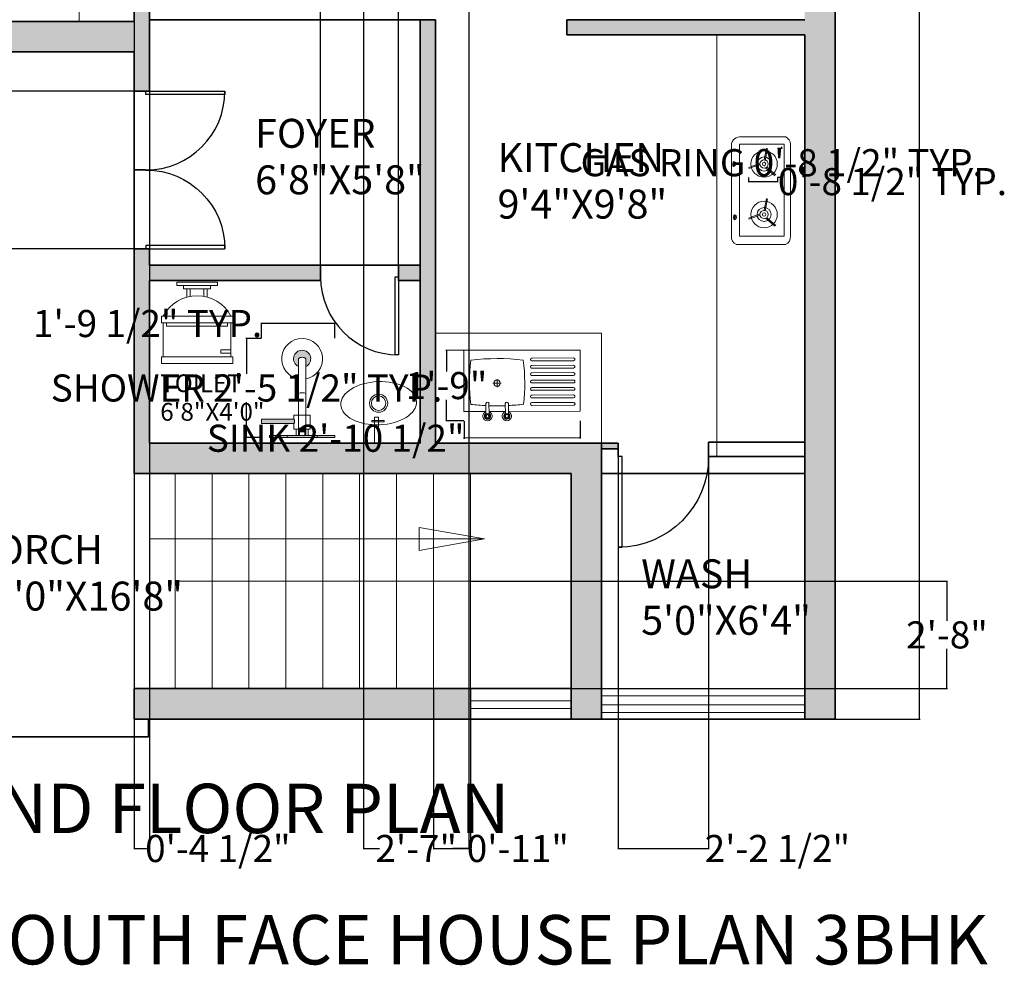
# Model space of a CAD drawing. Units: inches. Extents: x -4737294 to -4736756, y 1716389 to 1717040.
# Tile 16 of 25: x -4737096 to -4736805, y 1716389 to 1716669. Entities that reach past the tile are written whole.
import ezdxf

# ---------------------------------------------------------------- set-up
doc = ezdxf.new("R2010")
doc.units = ezdxf.units.IN
doc.header["$MEASUREMENT"] = 0
for name, color, linetype, lineweight in [('A-ANNO-DIMS', 2, 'Continuous', 18), ('A-ANNO-TEXT', 250, 'Continuous', 30), ('A-AREA-IDEN', 250, 'Continuous', 18), ('A-EQPM', 250, 'Continuous', 18), ('A-FLOR-CASE', 250, 'Continuous', 18), ('A-FLOR-STRS', 252, 'Continuous', 18), ('A-GLAZ', 4, 'Continuous', 18), ('A-WALL-PATT', 244, 'Continuous', 13), ('doors', 252, 'Continuous', 25), ('furniture', 250, 'Continuous', 18), ('PLUMBING FIXTURES', 252, 'Continuous', 18), ('walls', 252, 'Continuous', 35)]:
    doc.layers.add(name, color=color, linetype=linetype, lineweight=lineweight)
doc.styles.get("Standard").update_dxf_attribs({"font": 'arial.ttf'})
doc.dimstyles.get("Standard").update_dxf_attribs({"dimtxt": 8, "dimasz": 0.18, "dimexe": 0.18, "dimexo": 0.0625, "dimgap": 0.09, "dimtad": 0, "dimtih": 1, "dimtoh": 1, "dimzin": 0, "dimdsep": 46, "dimlunit": 3, "dimtxsty": 'Standard', "dimcen": 0.09, "dimadec": 0, "dimazin": 0, "dimtfac": 1, "dimtofl": 0, "dimtmove": 0, "dimatfit": 3, "dimfxl": 1, "dimtolj": 1, "dimtzin": 0, "dimarcsym": 0})

# ---------------------------------------------------------------- blocks, each defined once
blk = doc.blocks.new('*D22')
at = {"layer": 'A-ANNO-DIMS', "color": 0, "lineweight": -2, "transparency": 16777216}
for p, q in [((-4736855.08, 1717002.06), (-4736830.06, 1717002.06)), ((-4736830.24, 1717001.88), (-4736830.24, 1716736.22)), ((-4736830.24, 1716462.24), (-4736830.24, 1716727.91)), ((-4736855.08, 1716462.06), (-4736830.06, 1716462.06))]:
    blk.add_line(p, q, dxfattribs=at)
at = {"layer": 'A-ANNO-DIMS', "color": 0, "transparency": 16777216}
for points in [[(-4736830.27, 1717001.88), (-4736830.21, 1717001.88), (-4736830.24, 1717002.06)], [(-4736830.27, 1716462.24), (-4736830.21, 1716462.24), (-4736830.24, 1716462.06)]]:
    blk.add_solid(points, dxfattribs=at)
at = {"layer": 'Defpoints', "color": 0, "transparency": 16777216}
for p in [(-4736855.14, 1717002.06), (-4736830.24, 1717002.06), (-4736855.14, 1716462.06)]:
    blk.add_point(p, dxfattribs=at)
at = {"layer": 'A-ANNO-DIMS', "color": 0, "transparency": 16777216, "insert": (-4736830.24, 1716732.06), "char_height": 8, "attachment_point": 5}
blk.add_mtext("\\A1;45'", dxfattribs=at)
blk = doc.blocks.new('A$C799204C7')
for p, q in [((0, 34.2), (17.99, 34.2)), ((0, 0), (0, 34.2)), ((2.32, 20.01), (2.32, 32.27)), ((3.13, 20.01), (3.13, 32.27)), ((4.48, 20.01), (4.48, 32.27)), ((5.29, 20.01), (5.29, 32.27)), ((6.64, 20.01), (6.64, 32.27)), ((7.45, 20.01), (7.45, 32.27)), ((8.85, 20.01), (8.85, 32.27)), ((9.66, 20.01), (9.66, 32.27)), ((11.01, 20.01), (11.01, 32.27)), ((11.82, 20.01), (11.82, 32.27)), ((13.22, 20.01), (13.22, 32.27)), ((14.03, 20.01), (14.03, 32.27)), ((15.42, 20.01), (15.42, 32.27)), ((16.24, 20.01), (16.24, 32.27)), ((17.99, 13.08), (17.99, 34.2)), ((18.59, 13.08), (15.71, 13.08)), ((15.71, 12.17), (18.59, 12.17)), ((17.99, 7.36), (17.99, 12.17)), ((8.52, 9.77), (10.9, 9.77)), ((9.73, 11), (9.73, 8.54)), ((18.59, 7.36), (15.71, 7.36)), ((15.71, 6.45), (18.59, 6.45)), ((17.99, 0), (17.99, 6.45)), ((0, 0), (17.99, 0))]:
    blk.add_line(p, q)
for centre, radius in [((19.38, 12.62), 0.684), ((19.38, 12.62), 0.456), ((9.7, 9.77), 0.916), ((19.38, 6.91), 0.684), ((19.38, 6.91), 0.456)]:
    blk.add_circle(centre, radius)
for centre, radius, start, end in [((2.72, 32.27), 0.407, 0, 180), ((4.88, 32.27), 0.407, 0, 180), ((7.05, 32.27), 0.407, 0, 180), ((9.25, 32.27), 0.407, 0, 180), ((11.42, 32.27), 0.407, 0, 180), ((13.62, 32.27), 0.407, 0, 180), ((15.83, 32.27), 0.407, 0, 180), ((2.72, 20.01), 0.407, 180, 0), ((67.33, 9.77), 64.88, 173.1952, 186.8048), ((9.53, -30.19), 48.1, 82.3437, 97.8966), ((4.88, 20.01), 0.407, 180, 0), ((7.05, 20.01), 0.407, 180, 0), ((9.25, 20.01), 0.407, 180, 0), ((11.42, 20.01), 0.407, 180, 0), ((13.62, 20.01), 0.407, 180, 0), ((15.83, 20.01), 0.407, 180, 0), ((-48.51, 9.77), 64.88, 2.9208, 6.8048), ((15.71, 12.62), 0.456, 90, 270), ((-48.51, 9.77), 64.88, 357.8723, 2.115), ((19.38, 12.62), 1.37, 199.6514, 160.3603), ((19.38, 12.62), 0.911, 210.3431, 149.7554), ((15.71, 6.91), 0.456, 90, 270), ((-48.51, 9.77), 64.88, 353.1952, 357.0665), ((19.38, 6.91), 1.37, 199.6514, 160.3603), ((19.38, 6.91), 0.911, 210.3431, 149.7554), ((9.53, 49.73), 48.1, 262.1034, 277.6563)]:
    blk.add_arc(centre, radius, start, end)
blk = doc.blocks.new('sink')
at = {"layer": 'furniture'}
for p, q in [((8718164202.684322, -1433730581.131674), (8718164202.684322, -1433730583.598095)), ((8718164203.894819, -1433730582.369047), (8718164201.504578, -1433730582.369047)), ((8718164196.150837, -1433730592.638258), (8718164196.150837, -1433730604.938997)), ((8718164196.967728, -1433730592.638258), (8718164196.967728, -1433730604.938997)), ((8718164198.365185, -1433730592.638258), (8718164198.365185, -1433730604.938997)), ((8718164199.182076, -1433730592.638258), (8718164199.182076, -1433730604.938997)), ((8718164200.579533, -1433730592.638258), (8718164200.579533, -1433730604.938997)), ((8718164201.396423, -1433730592.638258), (8718164201.396423, -1433730604.938997)), ((8718164202.748692, -1433730592.638258), (8718164202.748692, -1433730604.938997)), ((8718164203.565582, -1433730592.638258), (8718164203.565582, -1433730604.938997)), ((8718164204.963041, -1433730592.638258), (8718164204.963041, -1433730604.938997)), ((8718164205.779934, -1433730592.638258), (8718164205.779934, -1433730604.938997)), ((8718164207.1322, -1433730592.638258), (8718164207.1322, -1433730604.938997)), ((8718164207.949093, -1433730592.638258), (8718164207.949093, -1433730604.938997)), ((8718164209.301359, -1433730592.638258), (8718164209.301359, -1433730604.938997)), ((8718164210.118252, -1433730592.638258), (8718164210.118252, -1433730604.938997))]:
    blk.add_line(p, q, dxfattribs=at)
for centre, radius in [((8718164192.998869, -1433730579.495552), 0.685789), ((8718164192.998869, -1433730579.495552), 0.457192), ((8718164202.715019, -1433730582.369047), 0.919003), ((8718164192.998869, -1433730585.228166), 0.68579), ((8718164192.998869, -1433730585.228166), 0.68579), ((8718164192.998869, -1433730585.228166), 0.457192)]:
    blk.add_circle(centre, radius, dxfattribs=at)
for centre, radius, start, end in [((8718164196.559284, -1433730592.638258), 0.41045, 354.3355999, 185.6644001), ((8718164198.77363, -1433730592.638258), 0.41045, 354.3355999, 185.6644001), ((8718164200.98798, -1433730592.638258), 0.41045, 354.3355999, 185.6644001), ((8718164203.157139, -1433730592.638258), 0.41045, 354.3355999, 185.6644001), ((8718164205.371487, -1433730592.638258), 0.41045, 354.3355999, 185.6644001), ((8718164207.540646, -1433730592.640262), 0.41045, 354.3355999, 185.6644001), ((8718164209.709805, -1433730592.640262), 0.41045, 354.3355999, 185.6644001), ((8718164196.559284, -1433730604.938997), 0.408445, 180, 0), ((8718164198.77363, -1433730604.938997), 0.408445, 180, 0), ((8718164200.98798, -1433730604.938997), 0.408445, 180, 0), ((8718164203.157139, -1433730604.938997), 0.408445, 180, 0), ((8718164205.371487, -1433730604.938997), 0.408445, 180, 0), ((8718164207.540646, -1433730604.938997), 0.408445, 180, 0), ((8718164209.709805, -1433730604.938997), 0.408445, 180, 0)]:
    blk.add_arc(centre, radius, start, end, dxfattribs=at)
at = {"layer": 'furniture', "xscale": 1.0032, "yscale": 1.0032, "zscale": 1.0032, "rotation": 180}
blk.add_blockref('A$C799204C7', (8718164212.441259, -1433730572.566334), dxfattribs=at)
blk = doc.blocks.new('washbasin')
at = {"layer": 'furniture'}
blk.add_blockref('sink', (-8718164214.119328, 1433730589.721069), dxfattribs=at)
blk = doc.blocks.new('O.H SHOWER-PL')
at = {"layer": 'PLUMBING FIXTURES'}
for points in [[(-1.84, 0), (-1.84, -0.25), (1.84, -0.25), (1.84, 0)], [(0.46, -8.72), (0.46, -9.67, -0.422337), (-0.46, -9.67), (-0.46, -8.72, 4.325472)]]:
    blk.add_hatch(color=256, dxfattribs=at).paths.add_polyline_path(points)
for p, q in [((-1.84, 0), (-1.84, -0.25)), ((1.84, 0), (-1.84, 0)), ((1.84, 0), (1.84, -0.25)), ((1.84, -0.25), (-1.84, -0.25)), ((-0.46, -0.25), (-0.46, -9.67)), ((0.46, -0.25), (0.46, -9.67))]:
    blk.add_line(p, q, dxfattribs=at)
for centre, radius, start, end in [((0, -4.48), 1.03, 243.53, 296.47), ((0, -9.67), 2.5, 100.61, 79.39), ((0, -9.67), 1.05, 116.0349, 63.9652), ((0, -9.22), 0.643, 224.2078, 315.7922)]:
    blk.add_arc(centre, radius, start, end, dxfattribs=at)
blk = doc.blocks.new('DIVERTER-PL')
at = {"layer": 'PLUMBING FIXTURES'}
for points in [[(4, 0), (-4, 0), (-4, -0.25), (4, -0.25)], [(0.38, -1.14), (0.38, -0.7), (-0.37, -0.7), (-0.37, -1.14)], [(1, -1.75, 0.30818), (1, -2.25), (5, -2.25), (5, -1.75)]]:
    blk.add_hatch(color=256, dxfattribs=at).paths.add_polyline_path(points)
for p, q in [((-4, 0), (-4, -0.25)), ((-4, 0), (4, 0)), ((4, 0), (4, -0.25)), ((-4, -0.25), (4, -0.25)), ((-4, -0.25), (4, -0.25)), ((-1, -1.05), (-0.37, -1.05)), ((-1, -1.05), (-1, -2.75)), ((-0.75, -0.25), (-0.75, -1.05)), ((-0.37, -0.7), (0.38, -0.7)), ((-0.37, -0.7), (-0.37, -1.14)), ((-0.37, -1.14), (0.38, -1.14)), ((-0.32, -0.7), (-0.32, -0.25)), ((0.32, -0.7), (0.32, -0.25)), ((0.38, -0.7), (0.38, -1.14)), ((0.38, -1.05), (1, -1.05)), ((0.75, -0.25), (0.75, -1.05)), ((1, -1.05), (1, -1.75)), ((1, -2.25), (1, -2.75)), ((-1, -2.75), (1, -2.75))]:
    blk.add_line(p, q, dxfattribs=at)
at = {"layer": 'PLUMBING FIXTURES', "ltscale": 12}
for p, q in [((1, -1.75), (5, -1.75)), ((1, -2.25), (5, -2.25)), ((5, -2.25), (5, -1.75))]:
    blk.add_line(p, q, dxfattribs=at)
at = {"layer": 'PLUMBING FIXTURES'}
blk.add_arc((1.37, -2), 0.444, 145.7435, 214.2565, dxfattribs=at)
blk = doc.blocks.new('A$C7F153053')
at = {"layer": 'PLUMBING FIXTURES', "xscale": -1, "rotation": 270}
for name in ['DIVERTER-PL', 'O.H SHOWER-PL']:
    blk.add_blockref(name, (12.17, 4), dxfattribs=at)
blk = doc.blocks.new('Toilet - Imperial')
for p, q in [((-10, 22), (-10, 12)), ((-10, 21), (-7, 21)), ((-7, 21), (-7, 20)), ((10, 12), (10, 22)), ((-7, 20), (-10, 20)), ((10.5, 12), (-10.5, 12)), ((-10.5, 10), (-10.5, 12)), ((9, 13), (-9, 13)), ((-9, 13), (-9, 12)), ((9, 12), (9, 13)), ((10.5, 12), (10.5, 10)), ((10.5, 10), (-10.5, 10)), ((-3, 4.4065), (-3, 2)), ((-2, 2), (-2, 4.1658)), ((2, 4.1658), (2, 2)), ((3, 2), (3, 4.4065)), ((4, 2), (-4, 2)), ((-4, 2), (-4, 1)), ((4, 1), (4, 2))]:
    blk.add_line(p, q)
for points in [[(10.5, 22), (10.5, 24), (-10.5, 24), (-10.5, 22)], [(6, 0), (6, 1), (-6, 1), (-6, 0)]]:
    blk.add_lwpolyline(points, close=True)
blk.add_arc((0, 15.3333), 11.3333, 208.0725, 331.9275)
blk = doc.blocks.new('*U20')
for p, q in [((0, 0), (0, -6)), ((40, 0), (40, -6))]:
    blk.add_line(p, q)
blk.add_lwpolyline([(0, 0), (0, 40), (1.75, 40), (1.75, 0)], close=True)
blk.add_arc((0, 0), 40, 0, 90)
blk = doc.blocks.new('LAVATORY-OVAL-WITH-TAP')
for p, q in [((6.3, 12.81), (6.3, 9.15)), ((6.71, 12.81), (6.3, 12.81)), ((6.71, 9.15), (6.71, 12.81)), ((0, 11.19), (7.64, 11.19)), ((7.64, 9.95), (0, 9.95)), ((6.3, 9.15), (6.71, 9.15)), ((7.64, 11.19), (7.64, 9.95))]:
    blk.add_line(p, q)
for radius in [2.67, 2.13, 2.13, 2.13]:
    blk.add_circle((11.77, 11.19), radius)
blk.add_ellipse((11.77, 11.19), major_axis=(-0.46, -11.19), ratio=0.56899)
blk = doc.blocks.new('COOKTOP-GAS-BURNER')
for p, q in [((4.61, 5.14), (5.29, 8.59)), ((4.94, 4.96), (5.59, 8.52)), ((3.4, 4.08), (0, 2.86)), ((3.41, 3.71), (0.09, 2.57)), ((5.39, 2.97), (8.04, 0.66)), ((5.07, 2.78), (7.83, 0.44))]:
    blk.add_line(p, q)
for radius in [3.91, 2.08, 1.22, 0.507]:
    blk.add_circle((4.61, 3.91), radius)
blk = doc.blocks.new('*D29')
at = {"layer": 'A-ANNO-DIMS', "color": 0, "lineweight": -2, "transparency": 16777216}
for p, q in [((-4737024.63, 1716574.47), (-4737029.14, 1716574.47)), ((-4737028.96, 1716574.29), (-4737028.96, 1716564.05)), ((-4737028.96, 1716545.37), (-4737028.96, 1716555.6)), ((-4737024.63, 1716545.19), (-4737029.14, 1716545.19))]:
    blk.add_line(p, q, dxfattribs=at)
at = {"layer": 'A-ANNO-DIMS', "color": 0, "transparency": 16777216}
for points in [[(-4737028.99, 1716574.29), (-4737028.93, 1716574.29), (-4737028.96, 1716574.47)], [(-4737028.99, 1716545.37), (-4737028.93, 1716545.37), (-4737028.96, 1716545.19)]]:
    blk.add_solid(points, dxfattribs=at)
at = {"layer": 'Defpoints', "color": 0, "transparency": 16777216}
for p in [(-4737024.57, 1716574.47), (-4737028.96, 1716545.19), (-4737024.57, 1716545.19)]:
    blk.add_point(p, dxfattribs=at)
at = {"layer": 'A-ANNO-DIMS', "color": 0, "transparency": 16777216, "insert": (-4737028.96, 1716559.83), "char_height": 8, "attachment_point": 5}
blk.add_mtext('\\A1;SHOWER 2\'-5 1/2" TYP.', dxfattribs=at)
blk = doc.blocks.new('*D30')
at = {"layer": 'A-ANNO-DIMS', "color": 0, "lineweight": -2, "transparency": 16777216}
for p, q in [((-4737024.57, 1716574.53), (-4737024.57, 1716579.04)), ((-4737002.91, 1716574.53), (-4737002.91, 1716579.04)), ((-4737024.57, 1716578.86), (-4737024.75, 1716578.86)), ((-4737003.09, 1716578.86), (-4737024.39, 1716578.86))]:
    blk.add_line(p, q, dxfattribs=at)
at = {"layer": 'A-ANNO-DIMS', "color": 0, "transparency": 16777216}
for points in [[(-4737024.39, 1716578.89), (-4737024.39, 1716578.83), (-4737024.57, 1716578.86)], [(-4737003.09, 1716578.89), (-4737003.09, 1716578.83), (-4737002.91, 1716578.86)]]:
    blk.add_solid(points, dxfattribs=at)
at = {"layer": 'Defpoints', "color": 0, "transparency": 16777216}
for p in [(-4737024.57, 1716578.86), (-4737024.57, 1716574.47), (-4737002.91, 1716574.47)]:
    blk.add_point(p, dxfattribs=at)
at = {"layer": 'A-ANNO-DIMS', "color": 0, "transparency": 16777216, "insert": (-4737058.17, 1716578.86), "char_height": 8, "attachment_point": 5}
blk.add_mtext('\\A1;1\'-9 1/2" TYP.', dxfattribs=at)
blk = doc.blocks.new('*D49')
at = {"layer": 'A-ANNO-DIMS', "color": 0, "lineweight": -2, "transparency": 16777216}
for p, q in [((-4736872.16, 1716630.64), (-4736870.76, 1716630.64)), ((-4736870.94, 1716630.82), (-4736870.94, 1716631)), ((-4736872.16, 1716622.06), (-4736870.76, 1716622.06)), ((-4736870.94, 1716621.88), (-4736870.94, 1716621.7))]:
    blk.add_line(p, q, dxfattribs=at)
at = {"layer": 'A-ANNO-DIMS', "color": 0, "transparency": 16777216}
for points in [[(-4736870.97, 1716630.82), (-4736870.91, 1716630.82), (-4736870.94, 1716630.64)], [(-4736870.97, 1716621.88), (-4736870.91, 1716621.88), (-4736870.94, 1716622.06)]]:
    blk.add_solid(points, dxfattribs=at)
at = {"layer": 'Defpoints', "color": 0, "transparency": 16777216}
for p in [(-4736872.23, 1716630.64), (-4736870.94, 1716630.64), (-4736872.23, 1716622.06)]:
    blk.add_point(p, dxfattribs=at)
at = {"layer": 'A-ANNO-DIMS', "color": 0, "transparency": 16777216, "insert": (-4736870.94, 1716626.35), "char_height": 8, "attachment_point": 5}
blk.add_mtext('\\A1;GAS RING 0\'-8 1/2" TYP.', dxfattribs=at)
blk = doc.blocks.new('*D50')
at = {"layer": 'A-ANNO-DIMS', "color": 0, "lineweight": -2, "transparency": 16777216}
for p, q in [((-4736880.75, 1716621.99), (-4736880.75, 1716620.59)), ((-4736880.57, 1716620.77), (-4736872.41, 1716620.77)), ((-4736872.23, 1716621.99), (-4736872.23, 1716620.59)), ((-4736872.23, 1716620.77), (-4736872.05, 1716620.77))]:
    blk.add_line(p, q, dxfattribs=at)
at = {"layer": 'A-ANNO-DIMS', "color": 0, "transparency": 16777216}
for points in [[(-4736880.57, 1716620.8), (-4736880.57, 1716620.74), (-4736880.75, 1716620.77)], [(-4736872.41, 1716620.8), (-4736872.41, 1716620.74), (-4736872.23, 1716620.77)]]:
    blk.add_solid(points, dxfattribs=at)
at = {"layer": 'Defpoints', "color": 0, "transparency": 16777216}
for p in [(-4736880.75, 1716622.06), (-4736872.23, 1716622.06), (-4736872.23, 1716620.77)]:
    blk.add_point(p, dxfattribs=at)
at = {"layer": 'A-ANNO-DIMS', "color": 0, "transparency": 16777216, "insert": (-4736838.25, 1716620.77), "char_height": 8, "attachment_point": 5}
blk.add_mtext('\\A1;0\'-8 1/2" TYP.', dxfattribs=at)
blk = doc.blocks.new('*D55')
at = {"layer": 'A-ANNO-DIMS', "color": 0, "lineweight": -2, "transparency": 16777216}
for p, q in [((-4736964.74, 1716550.08), (-4736964.73, 1716544.81)), ((-4736930.43, 1716550.15), (-4736930.42, 1716544.89)), ((-4736964.73, 1716544.99), (-4736964.91, 1716544.99)), ((-4736930.6, 1716545.07), (-4736964.55, 1716544.99))]:
    blk.add_line(p, q, dxfattribs=at)
at = {"layer": 'A-ANNO-DIMS', "color": 0, "transparency": 16777216}
for points in [[(-4736964.55, 1716545.02), (-4736964.55, 1716544.96), (-4736964.73, 1716544.99)], [(-4736930.6, 1716545.1), (-4736930.6, 1716545.04), (-4736930.42, 1716545.07)]]:
    blk.add_solid(points, dxfattribs=at)
at = {"layer": 'Defpoints', "color": 0, "transparency": 16777216}
for p in [(-4736964.74, 1716550.14), (-4736930.43, 1716550.21), (-4736964.73, 1716544.99)]:
    blk.add_point(p, dxfattribs=at)
at = {"layer": 'A-ANNO-DIMS', "color": 0, "transparency": 16777216, "insert": (-4737002.64, 1716544.99), "char_height": 8, "attachment_point": 5}
blk.add_mtext('\\A1;SINK 2\'-10 1/2"', dxfattribs=at)
blk = doc.blocks.new('*D56')
at = {"layer": 'A-ANNO-DIMS', "color": 0, "lineweight": -2, "transparency": 16777216}
for p, q in [((-4736964.85, 1716570.95), (-4736970.11, 1716570.94)), ((-4736969.93, 1716570.76), (-4736969.92, 1716564.71)), ((-4736969.89, 1716550.31), (-4736969.9, 1716556.36)), ((-4736964.81, 1716550.14), (-4736970.07, 1716550.13))]:
    blk.add_line(p, q, dxfattribs=at)
at = {"layer": 'A-ANNO-DIMS', "color": 0, "transparency": 16777216}
for points in [[(-4736969.9, 1716570.76), (-4736969.96, 1716570.76), (-4736969.93, 1716570.94)], [(-4736969.86, 1716550.31), (-4736969.92, 1716550.31), (-4736969.89, 1716550.13)]]:
    blk.add_solid(points, dxfattribs=at)
at = {"layer": 'Defpoints', "color": 0, "transparency": 16777216}
for p in [(-4736969.93, 1716570.94), (-4736964.79, 1716570.95), (-4736964.74, 1716550.14)]:
    blk.add_point(p, dxfattribs=at)
at = {"layer": 'A-ANNO-DIMS', "color": 0, "transparency": 16777216, "insert": (-4736969.91, 1716560.54), "char_height": 8, "attachment_point": 5}
blk.add_mtext('\\A1;1\'-9"', dxfattribs=at)
blk = doc.blocks.new('*D62')
at = {"layer": 'A-ANNO-DIMS', "color": 0, "lineweight": -2, "transparency": 16777216}
for p, q in [((-4737062.14, 1716849), (-4737062.14, 1716423.69)), ((-4737057.64, 1716849), (-4737057.64, 1716423.69)), ((-4737061.96, 1716423.87), (-4737057.82, 1716423.87)), ((-4737057.64, 1716423.87), (-4737057.46, 1716423.87))]:
    blk.add_line(p, q, dxfattribs=at)
at = {"layer": 'A-ANNO-DIMS', "color": 0, "transparency": 16777216}
for points in [[(-4737061.96, 1716423.9), (-4737061.96, 1716423.84), (-4737062.14, 1716423.87)], [(-4737057.82, 1716423.9), (-4737057.82, 1716423.84), (-4737057.64, 1716423.87)]]:
    blk.add_solid(points, dxfattribs=at)
at = {"layer": 'Defpoints', "color": 0, "transparency": 16777216}
for p in [(-4737062.14, 1716849.06), (-4737057.64, 1716849.06), (-4737057.64, 1716423.87)]:
    blk.add_point(p, dxfattribs=at)
at = {"layer": 'A-ANNO-DIMS', "color": 0, "transparency": 16777216, "insert": (-4737037.42, 1716423.87), "char_height": 8, "attachment_point": 5}
blk.add_mtext('\\A1;0\'-4 1/2"', dxfattribs=at)
blk = doc.blocks.new('*D63')
at = {"layer": 'A-ANNO-DIMS', "color": 0, "lineweight": -2, "transparency": 16777216}
for p, q in [((-4737062.21, 1716647.49), (-4737270.32, 1716647.49)), ((-4737270.14, 1716647.31), (-4737270.14, 1716628.42)), ((-4737270.14, 1716601.06), (-4737270.14, 1716619.96)), ((-4737062.21, 1716600.88), (-4737270.32, 1716600.88))]:
    blk.add_line(p, q, dxfattribs=at)
at = {"layer": 'A-ANNO-DIMS', "color": 0, "transparency": 16777216}
for points in [[(-4737270.17, 1716647.31), (-4737270.11, 1716647.31), (-4737270.14, 1716647.49)], [(-4737270.17, 1716601.06), (-4737270.11, 1716601.06), (-4737270.14, 1716600.88)]]:
    blk.add_solid(points, dxfattribs=at)
at = {"layer": 'Defpoints', "color": 0, "transparency": 16777216}
for p in [(-4737270.14, 1716647.49), (-4737062.14, 1716647.49), (-4737062.14, 1716600.88)]:
    blk.add_point(p, dxfattribs=at)
at = {"layer": 'A-ANNO-DIMS', "color": 0, "transparency": 16777216, "insert": (-4737270.14, 1716624.19), "char_height": 8, "attachment_point": 5}
blk.add_mtext('\\A1;3\'-10 1/2"', dxfattribs=at)
blk = doc.blocks.new('*D64')
at = {"layer": 'A-ANNO-DIMS', "color": 0, "lineweight": -2, "transparency": 16777216}
for p, q in [((-4736994.45, 1716844.5), (-4736994.45, 1716423.69)), ((-4736963.28, 1716844.5), (-4736963.28, 1716423.69)), ((-4736994.27, 1716423.87), (-4736989.65, 1716423.87)), ((-4736963.46, 1716423.87), (-4736968.07, 1716423.87))]:
    blk.add_line(p, q, dxfattribs=at)
at = {"layer": 'A-ANNO-DIMS', "color": 0, "transparency": 16777216}
for points in [[(-4736994.27, 1716423.9), (-4736994.27, 1716423.84), (-4736994.45, 1716423.87)], [(-4736963.46, 1716423.9), (-4736963.46, 1716423.84), (-4736963.28, 1716423.87)]]:
    blk.add_solid(points, dxfattribs=at)
at = {"layer": 'Defpoints', "color": 0, "transparency": 16777216}
for p in [(-4736994.45, 1716844.56), (-4736963.28, 1716844.56), (-4736963.28, 1716423.87)]:
    blk.add_point(p, dxfattribs=at)
at = {"layer": 'A-ANNO-DIMS', "color": 0, "transparency": 16777216, "insert": (-4736978.86, 1716423.87), "char_height": 8, "attachment_point": 5}
blk.add_mtext('\\A1;2\'-7"', dxfattribs=at)
blk = doc.blocks.new('*D65')
at = {"layer": 'A-ANNO-DIMS', "color": 0, "lineweight": -2, "transparency": 16777216}
for p, q in [((-4737007.1, 1716596.13), (-4737007.1, 1717035.24)), ((-4737006.92, 1717035.06), (-4736984.27, 1717035.06)), ((-4736984.09, 1716596.13), (-4736984.09, 1717035.24)), ((-4736984.09, 1717035.06), (-4736983.91, 1717035.06))]:
    blk.add_line(p, q, dxfattribs=at)
at = {"layer": 'A-ANNO-DIMS', "color": 0, "transparency": 16777216}
for points in [[(-4737006.92, 1717035.09), (-4737006.92, 1717035.03), (-4737007.1, 1717035.06)], [(-4736984.27, 1717035.09), (-4736984.27, 1717035.03), (-4736984.09, 1717035.06)]]:
    blk.add_solid(points, dxfattribs=at)
at = {"layer": 'Defpoints', "color": 0, "transparency": 16777216}
for p in [(-4736984.09, 1717035.06), (-4737007.1, 1716596.06), (-4736984.09, 1716596.06)]:
    blk.add_point(p, dxfattribs=at)
at = {"layer": 'A-ANNO-DIMS', "color": 0, "transparency": 16777216, "insert": (-4736970.46, 1717035.06), "char_height": 8, "attachment_point": 5}
blk.add_mtext('\\A1;1\'-11"', dxfattribs=at)
blk = doc.blocks.new('*D67')
at = {"layer": 'A-ANNO-DIMS', "color": 0, "lineweight": -2, "transparency": 16777216}
for p, q in [((-4736919.25, 1716543.5), (-4736919.25, 1716423.69)), ((-4736892.51, 1716543.75), (-4736892.51, 1716423.69)), ((-4736919.07, 1716423.87), (-4736892.69, 1716423.87)), ((-4736892.51, 1716423.87), (-4736892.33, 1716423.87))]:
    blk.add_line(p, q, dxfattribs=at)
at = {"layer": 'A-ANNO-DIMS', "color": 0, "transparency": 16777216}
for points in [[(-4736919.07, 1716423.9), (-4736919.07, 1716423.84), (-4736919.25, 1716423.87)], [(-4736892.69, 1716423.9), (-4736892.69, 1716423.84), (-4736892.51, 1716423.87)]]:
    blk.add_solid(points, dxfattribs=at)
at = {"layer": 'Defpoints', "color": 0, "transparency": 16777216}
for p in [(-4736919.25, 1716543.56), (-4736892.51, 1716543.81), (-4736892.51, 1716423.87)]:
    blk.add_point(p, dxfattribs=at)
at = {"layer": 'A-ANNO-DIMS', "color": 0, "transparency": 16777216, "insert": (-4736872.22, 1716423.87), "char_height": 8, "attachment_point": 5}
blk.add_mtext('\\A1;2\'-2 1/2"', dxfattribs=at)
blk = doc.blocks.new('*D68')
at = {"layer": 'A-ANNO-DIMS', "color": 0, "lineweight": -2, "transparency": 16777216}
for p, q in [((-4736962.81, 1716502.81), (-4736821.96, 1716502.81)), ((-4736822.14, 1716502.63), (-4736822.14, 1716491.11)), ((-4736822.14, 1716471.24), (-4736822.14, 1716482.77)), ((-4736962.81, 1716471.06), (-4736821.96, 1716471.06))]:
    blk.add_line(p, q, dxfattribs=at)
at = {"layer": 'A-ANNO-DIMS', "color": 0, "transparency": 16777216}
for points in [[(-4736822.17, 1716502.63), (-4736822.11, 1716502.63), (-4736822.14, 1716502.81)], [(-4736822.17, 1716471.24), (-4736822.11, 1716471.24), (-4736822.14, 1716471.06)]]:
    blk.add_solid(points, dxfattribs=at)
at = {"layer": 'Defpoints', "color": 0, "transparency": 16777216}
for p in [(-4736962.87, 1716502.81), (-4736962.87, 1716471.06), (-4736822.14, 1716471.06)]:
    blk.add_point(p, dxfattribs=at)
at = {"layer": 'A-ANNO-DIMS', "color": 0, "transparency": 16777216, "insert": (-4736822.14, 1716486.94), "char_height": 8, "attachment_point": 5}
blk.add_mtext('\\A1;2\'-8"', dxfattribs=at)
blk = doc.blocks.new('*D69')
at = {"layer": 'A-ANNO-DIMS', "color": 0, "lineweight": -2, "transparency": 16777216}
for p, q in [((-4736973.77, 1716471), (-4736973.77, 1716423.69)), ((-4736962.87, 1716471), (-4736962.87, 1716423.69)), ((-4736973.59, 1716423.87), (-4736963.05, 1716423.87)), ((-4736962.87, 1716423.87), (-4736962.69, 1716423.87))]:
    blk.add_line(p, q, dxfattribs=at)
at = {"layer": 'A-ANNO-DIMS', "color": 0, "transparency": 16777216}
for points in [[(-4736973.59, 1716423.9), (-4736973.59, 1716423.84), (-4736973.77, 1716423.87)], [(-4736963.05, 1716423.9), (-4736963.05, 1716423.84), (-4736962.87, 1716423.87)]]:
    blk.add_solid(points, dxfattribs=at)
at = {"layer": 'Defpoints', "color": 0, "transparency": 16777216}
for p in [(-4736973.77, 1716471.06), (-4736962.87, 1716471.06), (-4736962.87, 1716423.87)]:
    blk.add_point(p, dxfattribs=at)
at = {"layer": 'A-ANNO-DIMS', "color": 0, "transparency": 16777216, "insert": (-4736948.86, 1716423.87), "char_height": 8, "attachment_point": 5}
blk.add_mtext('\\A1;0\'-11"', dxfattribs=at)

msp = doc.modelspace()

# ---------------------------------------------------------------- hatches: boundary and pattern name
at = {"layer": 'A-WALL-PATT'}
h = msp.add_hatch(color=256, dxfattribs=at)
h.dxf.hatch_style = 1
h.paths.add_polyline_path([(-4737206.144, 1716844.565), (-4737110.144, 1716844.565), (-4737110.144, 1716823.907), (-4737105.644, 1716823.907), (-4737105.644, 1716844.565), (-4737098.44, 1716844.565), (-4737098.44, 1716849.065), (-4737206.144, 1716849.065), (-4737206.144, 1716993.065), (-4736864.144, 1716993.065), (-4736864.144, 1716849.065), (-4736963.275, 1716849.065), (-4736994.446, 1716849.065), (-4736997.144, 1716849.065), (-4736997.144, 1716844.565), (-4736864.144, 1716844.565), (-4736864.144, 1716668.565), (-4736934.391, 1716668.565), (-4736934.391, 1716664.065), (-4736864.144, 1716664.065), (-4736864.144, 1716462.065), (-4736855.144, 1716462.065), (-4736855.144, 1717002.065), (-4737215.144, 1717002.065), (-4737215.144, 1716462.065), (-4737206.144, 1716462.065), (-4737206.144, 1716659.065), (-4737062.144, 1716659.065), (-4737062.144, 1716647.493), (-4737057.644, 1716647.493), (-4737057.644, 1716796.565), (-4737071.812, 1716796.565), (-4737071.812, 1716792.065), (-4737070.805, 1716792.065), (-4737062.144, 1716792.065), (-4737062.144, 1716668.065), (-4737206.144, 1716668.065), (-4737206.144, 1716792.065), (-4737093.784, 1716792.065), (-4737093.784, 1716796.565), (-4737206.144, 1716796.565)])
h = msp.add_hatch(color=256, dxfattribs=at)
h.dxf.hatch_style = 1
h.paths.add_polyline_path([(-4737057.644, 1716600.884), (-4737062.144, 1716600.884), (-4737062.144, 1716534.565), (-4736933.144, 1716534.565), (-4736933.144, 1716462.065), (-4736924.144, 1716462.065), (-4736924.144, 1716543.565), (-4736973.144, 1716543.565), (-4736973.144, 1716668.565), (-4736977.644, 1716668.565), (-4736977.644, 1716543.565), (-4737057.644, 1716543.565), (-4737057.644, 1716591.565), (-4737007.073, 1716591.565), (-4737007.073, 1716596.065), (-4737057.644, 1716596.065)])
h.paths.add_polyline_path([(-4736962.872, 1716471.065), (-4737062.144, 1716471.065), (-4737062.144, 1716462.065), (-4736962.872, 1716462.065)], flags=17)
h.paths.add_polyline_path([(-4737161.883, 1716716.26), (-4737096.689, 1716716.26), (-4737096.689, 1716729.349), (-4737161.883, 1716729.349)], flags=9)
h.paths.add_polyline_path([(-4737161.912, 1716729.958), (-4737095.809, 1716729.958), (-4737095.809, 1716743.222), (-4737161.912, 1716743.222)], flags=9)
h.paths.add_polyline_path([(-4736943.842, 1716913.818), (-4736878.647, 1716913.818), (-4736878.647, 1716926.907), (-4736943.842, 1716926.907)], flags=9)
h.paths.add_polyline_path([(-4736943.871, 1716927.516), (-4736877.767, 1716927.516), (-4736877.767, 1716940.78), (-4736943.871, 1716940.78)], flags=9)
h = msp.add_hatch(color=256, dxfattribs=at)
h.dxf.hatch_style = 1
h.paths.add_polyline_path([(-4737105.644, 1716800.884), (-4737109.098, 1716800.884), (-4737110.144, 1716800.884), (-4737110.144, 1716796.565), (-4737105.644, 1716796.565)], flags=17)
h.paths.add_polyline_path([(-4736977.644, 1716596.065), (-4736984.094, 1716596.065), (-4736984.094, 1716592.614), (-4736984.094, 1716591.565), (-4736977.644, 1716591.565)], flags=17)
h.paths.add_polyline_path([(-4736919.247, 1716543.565), (-4736924.144, 1716543.565), (-4736924.144, 1716541.852), (-4736919.247, 1716541.852)], flags=17)
h.paths.add_polyline_path([(-4737063.149, 1716767.883), (-4737063.149, 1716696.117), (-4737078.363, 1716696.117), (-4737078.363, 1716767.883)], flags=0)
h.paths.add_polyline_path([(-4737067.067, 1716762.706), (-4737067.067, 1716743.853), (-4737065.246, 1716743.853, -0.4142136), (-4737064.167, 1716742.774), (-4737064.167, 1716721.73, -0.4142136), (-4737065.246, 1716720.65), (-4737067.067, 1716720.65), (-4737067.067, 1716701.798), (-4737068.518, 1716701.798, -0.0640419), (-4737070.693, 1716705.267), (-4737070.693, 1716720.65), (-4737071.064, 1716720.65, -0.4142136), (-4737072.143, 1716721.73), (-4737072.143, 1716742.774, -0.4142136), (-4737071.064, 1716743.853), (-4737070.693, 1716743.853), (-4737070.693, 1716759.237, -0.0640419), (-4737068.518, 1716762.706)], flags=0)
h.paths.add_polyline_path([(-4737129.14, 1716769.472), (-4737129.14, 1716693.886), (-4737160.657, 1716693.886), (-4737160.657, 1716701.381), (-4737189.495, 1716701.381), (-4737189.373, 1716688.681), (-4737203.937, 1716688.681), (-4737204.06, 1716701.381), (-4737204.06, 1716758.068), (-4737204.182, 1716770.768), (-4737189.618, 1716770.768), (-4737189.495, 1716758.068), (-4737160.657, 1716758.068), (-4737160.657, 1716769.472)], flags=0)
h.paths.add_polyline_path([(-4737184.679, 1716758.007), (-4737184.679, 1716747.779), (-4737192.22, 1716747.779), (-4737192.27, 1716747.71), (-4737192.27, 1716707.782), (-4737200.836, 1716707.782), (-4737200.836, 1716724.392), (-4737192.27, 1716724.392), (-4737192.27, 1716731.169), (-4737200.836, 1716731.169), (-4737200.836, 1716747.779), (-4737192.22, 1716747.779)], flags=0)
h.paths.add_polyline_path([(-4737192.212, 1716764.76, -1), (-4737201.588, 1716764.76, -1)], flags=0)
h.paths.add_polyline_path([(-4737192.089, 1716695.373, -1), (-4737201.466, 1716695.373, -1)], flags=0)
h.paths.add_polyline_path([(-4737161.883, 1716716.26), (-4737096.689, 1716716.26), (-4737096.689, 1716729.349), (-4737161.883, 1716729.349)], flags=8)
h.paths.add_polyline_path([(-4737161.912, 1716729.958), (-4737095.809, 1716729.958), (-4737095.809, 1716743.222), (-4737161.912, 1716743.222)], flags=8)

# ---------------------------------------------------------------- linework, layer by layer
at = {"layer": 'A-EQPM'}
for p, q in [((-4736869.747, 1716633.988), (-4736883.37, 1716633.988)), ((-4736870.229, 1716631.846), (-4736883.37, 1716631.846)), ((-4736883.37, 1716631.846), (-4736883.37, 1716604.674)), ((-4736870.229, 1716604.674), (-4736870.229, 1716631.846)), ((-4736868.345, 1716631.846), (-4736868.345, 1716604.674)), ((-4736885.763, 1716630.911), (-4736885.763, 1716604.674)), ((-4736869.822, 1716602.227), (-4736884.357, 1716602.227)), ((-4736883.37, 1716604.674), (-4736870.229, 1716604.674))]:
    msp.add_line(p, q, dxfattribs=at)
for centre, radius, start, end in [((-4736883.19, 1716631.379), 2.615, 93.92707, 190.30452), ((-4736870.954, 1716631.667), 2.615, 3.92707, 62.5308), ((-4736883.373, 1716604.42), 2.404, 173.93636, 246.89401), ((-4736870.738, 1716604.45), 2.404, 292.40616, 5.36382)]:
    msp.add_arc(centre, radius, start, end, dxfattribs=at)
for centre, major_axis, ratio in [((-4736885.142, 1716625.971), (0.02, 0.713), 0.3769734), ((-4736884.873, 1716625.963), (0.043, 0.664), 0.4928397), ((-4736884.915, 1716610.201), (0.02, 0.713), 0.3769734), ((-4736884.646, 1716610.193), (0.043, 0.664), 0.4928397)]:
    msp.add_ellipse(centre, major_axis=major_axis, ratio=ratio, dxfattribs=at)
at = {"layer": 'A-FLOR-CASE'}
for p, q in [((-4736890.121, 1716539.554), (-4736890.121, 1716664.065)), ((-4736924.144, 1716575.986), (-4736973.144, 1716575.986)), ((-4736924.144, 1716543.565), (-4736924.144, 1716575.986))]:
    msp.add_line(p, q, dxfattribs=at)
at = {"layer": 'A-FLOR-STRS'}
for p, q in [((-4737050.019, 1716471.065), (-4737050.019, 1716534.565)), ((-4737039.125, 1716471.065), (-4737039.125, 1716534.565)), ((-4737028.232, 1716471.065), (-4737028.232, 1716534.565)), ((-4737017.339, 1716471.065), (-4737017.339, 1716534.565)), ((-4737006.446, 1716471.065), (-4737006.446, 1716534.565)), ((-4736995.552, 1716471.065), (-4736995.552, 1716534.565)), ((-4736984.659, 1716471.065), (-4736984.659, 1716534.565)), ((-4736973.766, 1716471.065), (-4736973.766, 1716534.565)), ((-4736962.872, 1716471.065), (-4736962.872, 1716534.565)), ((-4736978.02, 1716515.264), (-4736978.02, 1716518.682)), ((-4736978.02, 1716518.682), (-4736958.696, 1716515.264)), ((-4737057.337, 1716515.264), (-4736978.02, 1716515.264)), ((-4736978.02, 1716515.264), (-4736958.696, 1716515.264)), ((-4736978.02, 1716515.264), (-4736978.02, 1716511.846)), ((-4736978.02, 1716511.846), (-4736958.696, 1716515.264)), ((-4737050.019, 1716502.815), (-4736962.872, 1716502.815))]:
    msp.add_line(p, q, dxfattribs=at)
at = {"layer": 'A-GLAZ'}
for p, q in [((-4736962.872, 1716471.065), (-4736962.872, 1716462.065)), ((-4736933.144, 1716471.065), (-4736962.872, 1716471.065)), ((-4736962.872, 1716471.065), (-4736962.872, 1716467.479)), ((-4736933.144, 1716462.065), (-4736933.144, 1716471.065)), ((-4736924.144, 1716468.933), (-4736864.144, 1716468.933)), ((-4736864.144, 1716468.933), (-4736864.144, 1716466.251)), ((-4736962.872, 1716467.479), (-4736933.144, 1716467.479)), ((-4736933.144, 1716467.479), (-4736933.144, 1716465.223)), ((-4736864.144, 1716466.251), (-4736924.144, 1716466.251)), ((-4736924.144, 1716466.251), (-4736924.144, 1716464.026)), ((-4736933.144, 1716465.223), (-4736962.872, 1716465.223)), ((-4736924.144, 1716464.026), (-4736864.144, 1716464.026)), ((-4736962.872, 1716462.065), (-4736933.144, 1716462.065))]:
    msp.add_line(p, q, dxfattribs=at)
at = {"layer": 'furniture'}
msp.add_line((-4737078.363, 1716696.117), (-4737078.363, 1716668.065), dxfattribs=at)
at = {"layer": 'walls'}
for p, q in [((-4736855.144, 1717002.065), (-4736855.144, 1716462.065)), ((-4737057.644, 1716647.493), (-4737057.644, 1716796.565)), ((-4737062.144, 1716668.065), (-4737062.144, 1716792.065)), ((-4737206.144, 1716668.065), (-4737062.144, 1716668.065)), ((-4737057.644, 1716668.565), (-4736973.144, 1716668.565)), ((-4736977.644, 1716543.565), (-4736977.644, 1716668.565)), ((-4736973.144, 1716543.565), (-4736973.144, 1716668.565)), ((-4736934.391, 1716668.565), (-4736864.144, 1716668.565)), ((-4736934.391, 1716668.565), (-4736934.391, 1716664.065)), ((-4736934.391, 1716664.065), (-4736864.144, 1716664.065)), ((-4736864.144, 1716664.065), (-4736864.144, 1716462.065)), ((-4737206.144, 1716659.065), (-4737062.144, 1716659.065)), ((-4737062.144, 1716534.565), (-4737062.144, 1716659.065)), ((-4737062.144, 1716647.493), (-4737057.644, 1716647.493)), ((-4737062.144, 1716600.884), (-4737057.644, 1716600.884)), ((-4737057.644, 1716596.065), (-4737057.644, 1716600.884)), ((-4737057.644, 1716596.065), (-4736977.644, 1716596.065)), ((-4737007.073, 1716591.565), (-4737007.073, 1716596.065)), ((-4736984.094, 1716591.565), (-4736984.094, 1716596.065)), ((-4737057.644, 1716591.565), (-4737007.073, 1716591.565)), ((-4737057.644, 1716543.565), (-4737057.644, 1716591.565)), ((-4737057.644, 1716543.565), (-4737057.644, 1716591.565)), ((-4736984.094, 1716591.565), (-4736977.644, 1716591.565)), ((-4737057.644, 1716543.565), (-4736977.644, 1716543.565)), ((-4736973.144, 1716543.565), (-4736924.144, 1716543.565)), ((-4736924.144, 1716543.565), (-4736924.144, 1716462.065)), ((-4736924.144, 1716543.565), (-4736919.247, 1716543.565)), ((-4736924.144, 1716541.852), (-4736919.247, 1716541.852)), ((-4736919.247, 1716541.852), (-4736919.247, 1716543.565)), ((-4736892.508, 1716543.814), (-4736892.508, 1716539.554)), ((-4736864.144, 1716543.814), (-4736892.508, 1716543.814)), ((-4736864.144, 1716539.554), (-4736864.144, 1716543.814)), ((-4736892.508, 1716539.554), (-4736892.508, 1716534.565)), ((-4736892.508, 1716539.554), (-4736864.144, 1716539.554)), ((-4737062.144, 1716534.565), (-4736933.144, 1716534.565)), ((-4736933.144, 1716534.565), (-4736933.144, 1716462.065)), ((-4736924.144, 1716534.565), (-4736864.144, 1716534.565)), ((-4736933.144, 1716471.065), (-4737062.144, 1716471.065)), ((-4737062.144, 1716462.065), (-4737062.144, 1716471.065)), ((-4736855.144, 1716462.065), (-4737062.144, 1716462.065)), ((-4737057.851, 1716456.869), (-4737057.851, 1716462.065)), ((-4737215.144, 1716456.869), (-4737062.144, 1716456.869)), ((-4737062.144, 1716456.869), (-4737057.851, 1716456.869))]:
    msp.add_line(p, q, dxfattribs=at)

# ---------------------------------------------------------------- block references
at = {"layer": 'A-EQPM'}
for p in [(-4736880.752, 1716622.055), (-4736880.752, 1716607.142)]:
    msp.add_blockref('COOKTOP-GAS-BURNER', p, dxfattribs=at)
at = {"layer": 'doors'}
for p, xscale, yscale, zscale, rotation in [((-4737058.649, 1716647.493), 0.5826086806699359, 0.5826086806699359, 0.5826086806699359, 270), ((-4737058.649, 1716600.884), -0.5826086806699359, 0.5826086806699359, 0.5826086806699359, 270), ((-4736984.094, 1716592.614), 0.5750671146789703, 0.5750671146789703, 0.5750671146789703, 180), ((-4736919.247, 1716539.554), -0.6684818809186152, 0.6684818809186152, 0.6684818809186152, 180)]:
    msp.add_blockref('*U20', p, dxfattribs=dict(at, xscale=xscale, yscale=yscale, zscale=zscale, rotation=rotation))
at = {"layer": 'PLUMBING FIXTURES'}
for name, p, rotation in [('Toilet - Imperial', (-4737043.548, 1716591.065), 180), ('washbasin', (-4736947.635, 1716572.669), 90.12017160754561)]:
    msp.add_blockref(name, p, dxfattribs=dict(at, rotation=rotation))
at = {"layer": 'PLUMBING FIXTURES', "xscale": -2.406230429091579, "yscale": 2.406230429091579, "zscale": 2.406230429091579, "rotation": 90}
msp.add_blockref('A$C7F153053', (-4737002.914, 1716574.46), dxfattribs=at)
at = {"layer": 'PLUMBING FIXTURES', "extrusion": (0, 0, -1), "zscale": -1, "rotation": 90.00000003478877}
msp.add_blockref('LAVATORY-OVAL-WITH-TAP', (4737001.138, 1716543.565), dxfattribs=at)

# ---------------------------------------------------------------- texts
at = {"layer": 'A-ANNO-TEXT'}
for s, p in [('GROUND FLOOR PLAN', (-4737157.681, 1716428.409)), ('30X45 SOUTH FACE HOUSE PLAN 3BHK', (-4737171.362, 1716389.643))]:
    msp.add_text(s, height=14.58777, dxfattribs=at).set_placement(p)
at = {"layer": 'A-AREA-IDEN'}
for s, height, p in [('FOYER', 8.5453, (-4737026.417, 1716630.744)), ('KITCHEN', 8.5453, (-4736954.847, 1716623.569)), ('6\'8"X5\'8"', 8.5453, (-4737026.417, 1716617.017)), ('9\'4"X9\'8"', 8.5453, (-4736954.847, 1716609.842)), ('TOILET', 5.248, (-4737054.434, 1716558.593)), ('6\'8"X4\'0"', 5.248, (-4737054.434, 1716550.163)), ('PORCH', 8.5453, (-4737110.743, 1716507.85)), ('WASH', 8.5453, (-4736912.422, 1716500.699)), ('12\'0"X16\'8"', 8.54529, (-4737110.743, 1716494.123)), ('5\'0"X6\'4"', 8.5453, (-4736912.422, 1716486.972))]:
    msp.add_text(s, height=height, dxfattribs=at).set_placement(p)

# ---------------------------------------------------------------- dimensions: what is measured, and where the dimension line sits
at = {"layer": 'A-ANNO-DIMS'}
for base, p1, p2, picture, middle in [((-4736984.094, 1717035.065), (-4737007.097, 1716596.065), (-4736984.094, 1716596.065), '*D65', (-4736970.46, 1717035.065)), ((-4737057.644, 1716423.869), (-4737062.144, 1716849.065), (-4737057.644, 1716849.065), '*D62', (-4737037.421, 1716423.869)), ((-4736963.275, 1716423.869), (-4736994.446, 1716844.565), (-4736963.275, 1716844.565), '*D64', (-4736978.861, 1716423.869)), ((-4736892.508, 1716423.869), (-4736919.247, 1716543.565), (-4736892.508, 1716543.814), '*D67', (-4736872.216, 1716423.869)), ((-4736962.872, 1716423.869), (-4736973.766, 1716471.065), (-4736962.872, 1716471.065), '*D69', (-4736948.862, 1716423.869))]:
    dim = msp.add_linear_dim(base=base, p1=p1, p2=p2, dimstyle='Standard', override={"dimdec": 1, "dimlfac": 1, "dimrnd": 0, "dimzin": 1, "dimdsep": 46, "dimlunit": 4, "dimfrac": 2}, dxfattribs=at)
    dim.commit()
    dim.dimension.update_dxf_attribs({"geometry": picture, "text_midpoint": middle})
for base, p1, p2, angle, override, picture, middle in [((-4736830.238, 1717002.065), (-4736855.144, 1716462.065), (-4736855.144, 1717002.065), 90, {"dimclrd": 0, "dimclre": 0, "dimclrt": 0}, '*D22', (-4736830.238, 1716732.065)), ((-4737270.144, 1716647.493), (-4737062.144, 1716600.884), (-4737062.144, 1716647.493), 90, {"dimdec": 1, "dimlfac": 1, "dimrnd": 0, "dimzin": 1, "dimdsep": 46, "dimlunit": 4, "dimfrac": 2}, '*D63', (-4737270.144, 1716624.188)), ((-4736969.933, 1716570.944), (-4736964.743, 1716550.141), (-4736964.786, 1716570.955), 90.12017, {"dimdec": 1, "dimlfac": 1, "dimrnd": 0, "dimzin": 1, "dimdsep": 46, "dimlunit": 4, "dimfrac": 2}, '*D56', (-4736969.911, 1716560.537)), ((-4736822.144166004, 1716471.064625001), (-4736962.872333999, 1716502.814625), (-4736962.872333999, 1716471.064625), 90, {"dimdec": 1, "dimlfac": 1, "dimrnd": 0, "dimzin": 1, "dimdsep": 46, "dimlunit": 4, "dimfrac": 2}, '*D68', (-4736822.144166003, 1716486.939625002))]:
    dim = msp.add_linear_dim(base=base, p1=p1, p2=p2, angle=angle, dimstyle='Standard', override=override, dxfattribs=at)
    dim.commit()
    dim.dimension.update_dxf_attribs({"geometry": picture, "text_midpoint": middle})
for base, p1, p2, angle, text, picture, middle in [((-4736870.937, 1716630.643), (-4736872.226, 1716622.055), (-4736872.226, 1716630.643), 90, 'GAS RING <> TYP.', '*D49', (-4736870.937, 1716626.349)), ((-4737024.57, 1716578.857), (-4737002.914, 1716574.465), (-4737024.57, 1716574.465), 180, '<> TYP.', '*D30', (-4737058.166, 1716578.857)), ((-4737028.962, 1716545.186), (-4737024.57, 1716574.465), (-4737024.57, 1716545.186), 270, 'SHOWER <> TYP.', '*D29', (-4737028.962, 1716559.826)), ((-4736964.732, 1716544.994), (-4736930.433, 1716550.213), (-4736964.743, 1716550.141), 180.12017, 'SINK <>', '*D55', (-4737002.639, 1716544.994))]:
    dim = msp.add_linear_dim(base=base, p1=p1, p2=p2, angle=angle, text=text, dimstyle='Standard', override={"dimdec": 1, "dimlfac": 1, "dimrnd": 0, "dimzin": 1, "dimdsep": 46, "dimlunit": 4, "dimfrac": 2}, dxfattribs=at)
    dim.commit()
    dim.dimension.update_dxf_attribs({"geometry": picture, "text_midpoint": middle})
dim = msp.add_linear_dim(base=(-4736872.226, 1716620.767), p1=(-4736880.752, 1716622.055), p2=(-4736872.226, 1716622.055), text='<> TYP.', dimstyle='Standard', override={"dimdec": 1, "dimlfac": 1, "dimrnd": 0, "dimzin": 1, "dimdsep": 46, "dimlunit": 4, "dimfrac": 2}, dxfattribs=at)
dim.commit()
dim.dimension.update_dxf_attribs({"geometry": '*D50', "text_midpoint": (-4736838.253, 1716620.767)})

doc.saveas('drawing.dxf')
